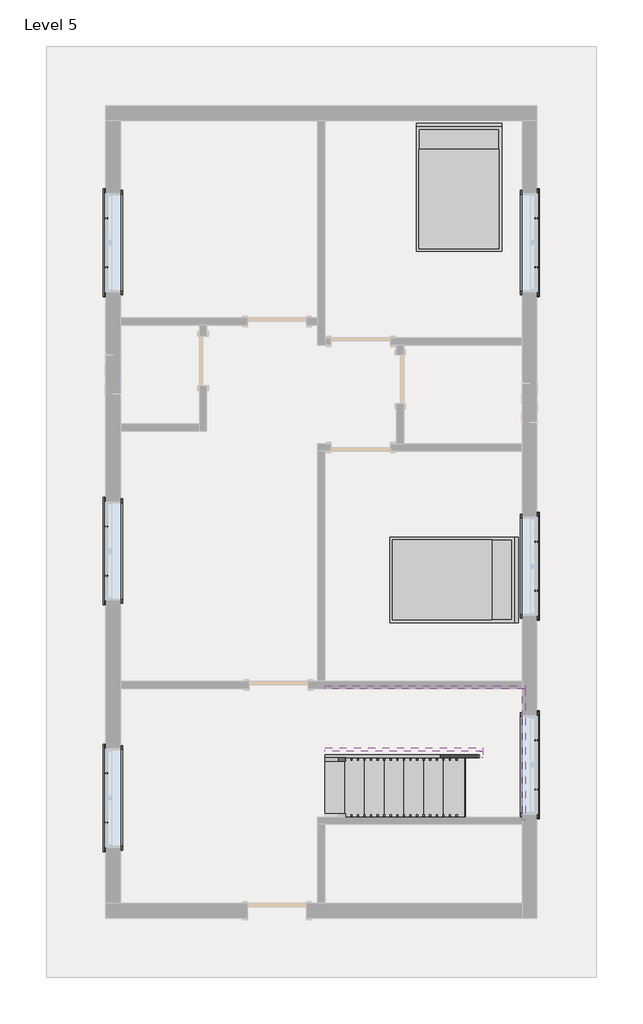
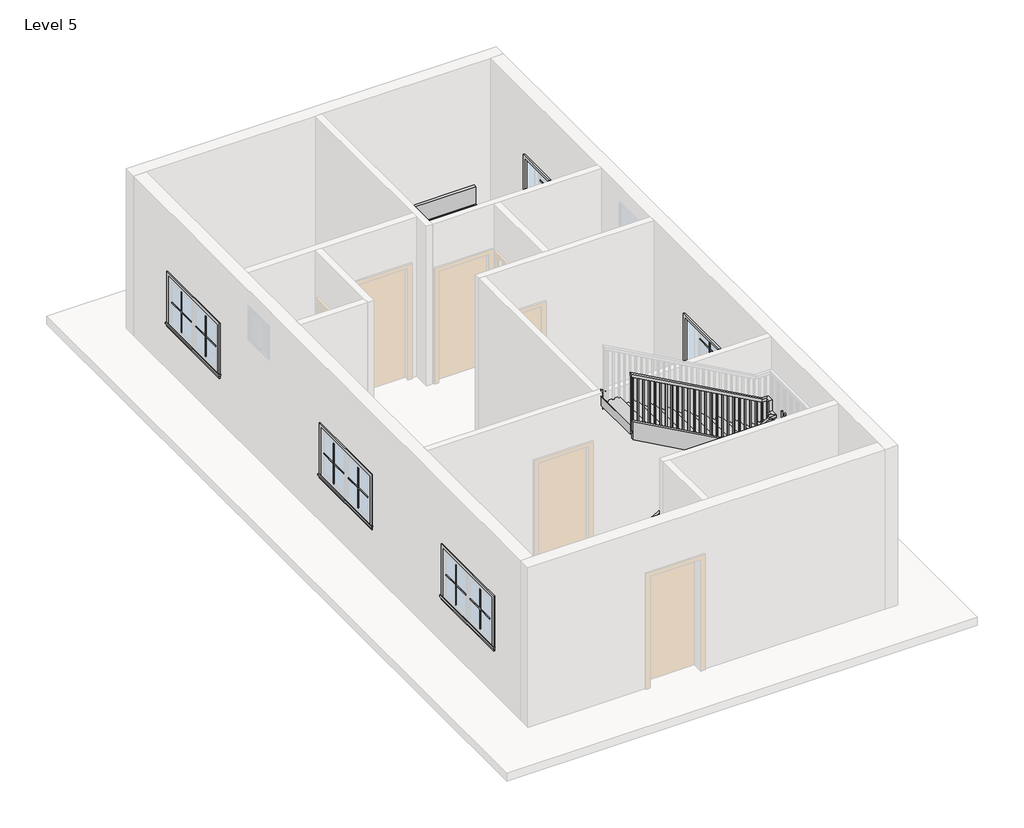
# One storey, part 3 of 3: 24 proxies, 6 members, 2 furniture elements, 1 railing, 1 stair flight.
"""IFC4 building model written with IfcOpenShell, lengths in millimetres."""

from ifc_helpers import new_model, si_unit, frame, origin, place, context, project, spatial, polyline, outline, extrude, faceted_brep, transform, mapped, element, save
from components import muntin_pattern_2x2_muntin_pattern_2x2_9352d081, muntin_pattern_2x2_muntin_pattern_2x2_5c2cbe28, trim_window_exterior_flat_with_sill_979bde60, trim_window_interior_flat_picture_frame_7883d11b, bed_17739_bed_17739_15c61121, stair_flight_c80fa3e3

model = new_model("IFC4")

# Units and contexts
model_context = context("Model", 3, world=origin())
ifc_project = project(units=[si_unit("LENGTHUNIT", "METRE", prefix="MILLI")], contexts=[model_context])

# Site, building, storey
site = spatial("IfcSite", under=ifc_project)
building = spatial("IfcBuilding", under=site)
storey = spatial("IfcBuildingStorey", under=building, Name="Level 5", Elevation=12649.2)

# Proxies
placement = place(None, origin())
muntin_pattern_2x2_muntin_pattern_2x2_shape = muntin_pattern_2x2_muntin_pattern_2x2_9352d081(model_context)
element("IfcBuildingElementProxy", 1, Name="Muntin Pattern_2x2 : Muntin Pattern_2x2", ObjectType="Muntin Pattern_2x2 : Muntin Pattern_2x2", at=placement, inside=storey, context=model_context, shape_type="MappedRepresentation", body=[
    mapped(muntin_pattern_2x2_muntin_pattern_2x2_shape, transform((-4579.34688, 3675.02881, 13633.45), x_axis=(0.0, 1.0, 0.0), y_axis=(-1.0, 0.0, 0.0), z_axis=(0.0, 0.0, 1.0))),
])
element("IfcBuildingElementProxy", 2, Name="Muntin Pattern_2x2 : Muntin Pattern_2x2", ObjectType="Muntin Pattern_2x2 : Muntin Pattern_2x2", at=placement, inside=storey, context=model_context, shape_type="MappedRepresentation", body=[
    mapped(muntin_pattern_2x2_muntin_pattern_2x2_shape, transform((-4579.34688, -1087.47119, 13633.45), x_axis=(0.0, 1.0, 0.0), y_axis=(-1.0, 0.0, 0.0), z_axis=(0.0, 0.0, 1.0))),
])
element("IfcBuildingElementProxy", 3, Name="Muntin Pattern_2x2 : Muntin Pattern_2x2", ObjectType="Muntin Pattern_2x2 : Muntin Pattern_2x2", at=placement, inside=storey, context=model_context, shape_type="MappedRepresentation", body=[
    mapped(muntin_pattern_2x2_muntin_pattern_2x2_shape, transform((-4579.34688, -4900.64619, 13633.45), x_axis=(0.0, 1.0, 0.0), y_axis=(-1.0, 0.0, 0.0), z_axis=(0.0, 0.0, 1.0))),
])
element("IfcBuildingElementProxy", 4, Name="Muntin Pattern_2x2 : Muntin Pattern_2x2", ObjectType="Muntin Pattern_2x2 : Muntin Pattern_2x2", at=placement, inside=storey, context=model_context, shape_type="MappedRepresentation", body=[
    mapped(muntin_pattern_2x2_muntin_pattern_2x2_shape, transform((2069.10312, -3630.64619, 13633.45), x_axis=(0.0, -1.0, 0.0), y_axis=(1.0, 0.0, 0.0), z_axis=(0.0, 0.0, 1.0))),
])
element("IfcBuildingElementProxy", 5, Name="Muntin Pattern_2x2 : Muntin Pattern_2x2", ObjectType="Muntin Pattern_2x2 : Muntin Pattern_2x2", at=placement, inside=storey, context=model_context, shape_type="MappedRepresentation", body=[
    mapped(muntin_pattern_2x2_muntin_pattern_2x2_shape, transform((2069.10312, 4433.85381, 13633.45), x_axis=(0.0, -1.0, 0.0), y_axis=(1.0, 0.0, 0.0), z_axis=(0.0, 0.0, 1.0))),
])
element("IfcBuildingElementProxy", 6, Name="Muntin Pattern_2x2 : Muntin Pattern_2x2", ObjectType="Muntin Pattern_2x2 : Muntin Pattern_2x2", at=placement, inside=storey, context=model_context, shape_type="MappedRepresentation", body=[
    mapped(muntin_pattern_2x2_muntin_pattern_2x2_shape, transform((2069.10312, -563.59619, 13633.45), x_axis=(0.0, -1.0, 0.0), y_axis=(1.0, 0.0, 0.0), z_axis=(0.0, 0.0, 1.0))),
])
muntin_pattern_2x2_muntin_pattern_2x2_2_shape = muntin_pattern_2x2_muntin_pattern_2x2_5c2cbe28(model_context)
element("IfcBuildingElementProxy", 7, Name="Muntin Pattern_2x2 : Muntin Pattern_2x2", ObjectType="Muntin Pattern_2x2 : Muntin Pattern_2x2", at=placement, inside=storey, context=model_context, shape_type="MappedRepresentation", body=[
    mapped(muntin_pattern_2x2_muntin_pattern_2x2_2_shape, transform((-4579.34688, 4433.85381, 13633.45), x_axis=(0.0, -1.0, 0.0), y_axis=(1.0, 0.0, 0.0), z_axis=(0.0, 0.0, 1.0))),
])
element("IfcBuildingElementProxy", 8, Name="Muntin Pattern_2x2 : Muntin Pattern_2x2", ObjectType="Muntin Pattern_2x2 : Muntin Pattern_2x2", at=placement, inside=storey, context=model_context, shape_type="MappedRepresentation", body=[
    mapped(muntin_pattern_2x2_muntin_pattern_2x2_2_shape, transform((-4579.34688, -328.64619, 13633.45), x_axis=(0.0, -1.0, 0.0), y_axis=(1.0, 0.0, 0.0), z_axis=(0.0, 0.0, 1.0))),
])
element("IfcBuildingElementProxy", 9, Name="Muntin Pattern_2x2 : Muntin Pattern_2x2", ObjectType="Muntin Pattern_2x2 : Muntin Pattern_2x2", at=placement, inside=storey, context=model_context, shape_type="MappedRepresentation", body=[
    mapped(muntin_pattern_2x2_muntin_pattern_2x2_2_shape, transform((-4579.34688, -4141.82119, 13633.45), x_axis=(0.0, -1.0, 0.0), y_axis=(1.0, 0.0, 0.0), z_axis=(0.0, 0.0, 1.0))),
])
element("IfcBuildingElementProxy", 10, Name="Muntin Pattern_2x2 : Muntin Pattern_2x2", ObjectType="Muntin Pattern_2x2 : Muntin Pattern_2x2", at=placement, inside=storey, context=model_context, shape_type="MappedRepresentation", body=[
    mapped(muntin_pattern_2x2_muntin_pattern_2x2_2_shape, transform((2069.10312, -4389.47119, 13633.45), x_axis=(0.0, 1.0, 0.0), y_axis=(-1.0, 0.0, 0.0), z_axis=(0.0, 0.0, 1.0))),
])
element("IfcBuildingElementProxy", 11, Name="Muntin Pattern_2x2 : Muntin Pattern_2x2", ObjectType="Muntin Pattern_2x2 : Muntin Pattern_2x2", at=placement, inside=storey, context=model_context, shape_type="MappedRepresentation", body=[
    mapped(muntin_pattern_2x2_muntin_pattern_2x2_2_shape, transform((2069.10312, 3675.02881, 13633.45), x_axis=(0.0, 1.0, 0.0), y_axis=(-1.0, 0.0, 0.0), z_axis=(0.0, 0.0, 1.0))),
])
element("IfcBuildingElementProxy", 12, Name="Muntin Pattern_2x2 : Muntin Pattern_2x2", ObjectType="Muntin Pattern_2x2 : Muntin Pattern_2x2", at=placement, inside=storey, context=model_context, shape_type="MappedRepresentation", body=[
    mapped(muntin_pattern_2x2_muntin_pattern_2x2_2_shape, transform((2069.10312, -1322.42119, 13633.45), x_axis=(0.0, 1.0, 0.0), y_axis=(-1.0, 0.0, 0.0), z_axis=(0.0, 0.0, 1.0))),
])
trim_window_exterior_flat_with_sill_shape = trim_window_exterior_flat_with_sill_979bde60(model_context)
element("IfcBuildingElementProxy", 13, Name="Trim-Window-Exterior-Flat : with Sill", ObjectType="Trim-Window-Exterior-Flat : with Sill", at=placement, inside=storey, context=model_context, shape_type="MappedRepresentation", body=[
    mapped(trim_window_exterior_flat_with_sill_shape, transform((-4588.87188, 4054.44131, 14478.0), x_axis=(0.0, -1.0, 0.0), y_axis=(0.0, 0.0, 1.0), z_axis=(-1.0, 0.0, 0.0))),
])
element("IfcBuildingElementProxy", 14, Name="Trim-Window-Exterior-Flat : with Sill", ObjectType="Trim-Window-Exterior-Flat : with Sill", at=placement, inside=storey, context=model_context, shape_type="MappedRepresentation", body=[
    mapped(trim_window_exterior_flat_with_sill_shape, transform((-4588.87188, -708.05869, 14478.0), x_axis=(0.0, -1.0, 0.0), y_axis=(0.0, 0.0, 1.0), z_axis=(-1.0, 0.0, 0.0))),
])
element("IfcBuildingElementProxy", 15, Name="Trim-Window-Exterior-Flat : with Sill", ObjectType="Trim-Window-Exterior-Flat : with Sill", at=placement, inside=storey, context=model_context, shape_type="MappedRepresentation", body=[
    mapped(trim_window_exterior_flat_with_sill_shape, transform((-4588.87188, -4521.23369, 14478.0), x_axis=(0.0, -1.0, 0.0), y_axis=(0.0, 0.0, 1.0), z_axis=(-1.0, 0.0, 0.0))),
])
element("IfcBuildingElementProxy", 16, Name="Trim-Window-Exterior-Flat : with Sill", ObjectType="Trim-Window-Exterior-Flat : with Sill", at=placement, inside=storey, context=model_context, shape_type="MappedRepresentation", body=[
    mapped(trim_window_exterior_flat_with_sill_shape, transform((2078.62812, -4010.05869, 14478.0), x_axis=(0.0, 1.0, 0.0), y_axis=(0.0, 0.0, 1.0), z_axis=(1.0, 0.0, 0.0))),
])
element("IfcBuildingElementProxy", 17, Name="Trim-Window-Exterior-Flat : with Sill", ObjectType="Trim-Window-Exterior-Flat : with Sill", at=placement, inside=storey, context=model_context, shape_type="MappedRepresentation", body=[
    mapped(trim_window_exterior_flat_with_sill_shape, transform((2078.62812, 4054.44131, 14478.0), x_axis=(0.0, 1.0, 0.0), y_axis=(0.0, 0.0, 1.0), z_axis=(1.0, 0.0, 0.0))),
])
element("IfcBuildingElementProxy", 18, Name="Trim-Window-Exterior-Flat : with Sill", ObjectType="Trim-Window-Exterior-Flat : with Sill", at=placement, inside=storey, context=model_context, shape_type="MappedRepresentation", body=[
    mapped(trim_window_exterior_flat_with_sill_shape, transform((2078.62812, -943.00869, 14478.0), x_axis=(0.0, 1.0, 0.0), y_axis=(0.0, 0.0, 1.0), z_axis=(1.0, 0.0, 0.0))),
])
trim_window_interior_flat_picture_frame_shape = trim_window_interior_flat_picture_frame_7883d11b(model_context)
element("IfcBuildingElementProxy", 19, Name="Trim-Window-Interior-Flat : Picture Frame", ObjectType="Trim-Window-Interior-Flat : Picture Frame", at=placement, inside=storey, context=model_context, shape_type="MappedRepresentation", body=[
    mapped(trim_window_interior_flat_picture_frame_shape, transform((-4360.27188, 4054.44131, 14478.0), x_axis=(0.0, 1.0, 0.0), y_axis=(0.0, 0.0, 1.0), z_axis=(1.0, 0.0, 0.0))),
])
element("IfcBuildingElementProxy", 20, Name="Trim-Window-Interior-Flat : Picture Frame", ObjectType="Trim-Window-Interior-Flat : Picture Frame", at=placement, inside=storey, context=model_context, shape_type="MappedRepresentation", body=[
    mapped(trim_window_interior_flat_picture_frame_shape, transform((-4360.27188, -708.05869, 14478.0), x_axis=(0.0, 1.0, 0.0), y_axis=(0.0, 0.0, 1.0), z_axis=(1.0, 0.0, 0.0))),
])
element("IfcBuildingElementProxy", 21, Name="Trim-Window-Interior-Flat : Picture Frame", ObjectType="Trim-Window-Interior-Flat : Picture Frame", at=placement, inside=storey, context=model_context, shape_type="MappedRepresentation", body=[
    mapped(trim_window_interior_flat_picture_frame_shape, transform((-4360.27188, -4521.23369, 14478.0), x_axis=(0.0, 1.0, 0.0), y_axis=(0.0, 0.0, 1.0), z_axis=(1.0, 0.0, 0.0))),
])
element("IfcBuildingElementProxy", 22, Name="Trim-Window-Interior-Flat : Picture Frame", ObjectType="Trim-Window-Interior-Flat : Picture Frame", at=placement, inside=storey, context=model_context, shape_type="MappedRepresentation", body=[
    mapped(trim_window_interior_flat_picture_frame_shape, transform((1850.02812, -4010.05869, 14478.0), x_axis=(0.0, -1.0, 0.0), y_axis=(0.0, 0.0, 1.0), z_axis=(-1.0, 0.0, 0.0))),
])
element("IfcBuildingElementProxy", 23, Name="Trim-Window-Interior-Flat : Picture Frame", ObjectType="Trim-Window-Interior-Flat : Picture Frame", at=placement, inside=storey, context=model_context, shape_type="MappedRepresentation", body=[
    mapped(trim_window_interior_flat_picture_frame_shape, transform((1850.02812, 4054.44131, 14478.0), x_axis=(0.0, -1.0, 0.0), y_axis=(0.0, 0.0, 1.0), z_axis=(-1.0, 0.0, 0.0))),
])
element("IfcBuildingElementProxy", 24, Name="Trim-Window-Interior-Flat : Picture Frame", ObjectType="Trim-Window-Interior-Flat : Picture Frame", at=placement, inside=storey, context=model_context, shape_type="MappedRepresentation", body=[
    mapped(trim_window_interior_flat_picture_frame_shape, transform((1850.02812, -943.00869, 14478.0), x_axis=(0.0, -1.0, 0.0), y_axis=(0.0, 0.0, 1.0), z_axis=(-1.0, 0.0, 0.0))),
])

# Furniture
bed_17739_bed_17739_shape = bed_17739_bed_17739_15c61121(model_context)
element("IfcFurniture", 25, ObjectType="Bed_17739 : Bed_17739", at=placement, inside=storey, context=model_context, shape_type="MappedRepresentation", body=[
    mapped(bed_17739_bed_17739_shape, transform((872.12812, 4886.29131, 12649.2), x_axis=(1.0, 0.0, 0.0), y_axis=(0.0, 1.0, 0.0), z_axis=(0.0, 0.0, 1.0))),
])
element("IfcFurniture", 26, ObjectType="Bed_17739 : Bed_17739", at=placement, inside=storey, context=model_context, shape_type="MappedRepresentation", body=[
    mapped(bed_17739_bed_17739_shape, transform((770.52812, -1152.55869, 12649.2), x_axis=(0.0, -1.0, 0.0), y_axis=(1.0, 0.0, 0.0), z_axis=(0.0, 0.0, 1.0))),
])

# Members
element("IfcMember", 27, ObjectType="Stringer - 2\" Width", at=placement, inside=storey, context=model_context, shape_type="SweptSolid", body=[
    extrude(outline(polyline([(12856.7983948, -1197.97188), (12649.2, -1197.97188), (12649.2, -944.0273772), (13834.5641651, 1189.62812), (14183.2428392, 1189.62812), (12856.7983948, -1197.97188)])), frame((0.0, -3902.10869, 0.0), z_axis=(0.0, 1.0, 0.0), x_axis=(0.0, 0.0, 1.0)), (0.0, 0.0, 1.0), 50.8),
])
element("IfcMember", 28, ObjectType="Stringer - 2\" Width", at=placement, inside=storey, context=model_context, shape_type="SweptSolid", body=[
    extrude(outline(polyline([(1240.42812, -3902.10869), (1189.62812, -3902.10869), (1189.62812, -3800.50869), (1240.42812, -3800.50869), (1240.42812, -3902.10869)])), frame((0.0, 0.0, 13944.6), z_axis=(0.0, 0.0, 1.0), x_axis=(1.0, 0.0, 0.0)), (0.0, 0.0, 1.0), 304.8),
])
element("IfcMember", 29, ObjectType="Stringer - 2\" Width", at=placement, inside=storey, context=model_context, shape_type="SweptSolid", body=[
    extrude(outline(polyline([(14032.1197207, 1240.42812), (14380.7983948, 1240.42812), (15735.4650614, -1197.97188), (15386.7863873, -1197.97188), (14032.1197207, 1240.42812)])), frame((0.0, -3800.50869, 0.0), z_axis=(0.0, 1.0, 0.0), x_axis=(0.0, 0.0, 1.0)), (0.0, 0.0, 1.0), 50.8),
])
element("IfcMember", 30, ObjectType="Stringer - 2\" Width", at=placement, inside=storey, context=model_context, shape_type="SweptSolid", body=[
    extrude(outline(polyline([(12856.7983948, -1197.97188), (12649.2, -1197.97188), (12649.2, -944.0273772), (14201.453054, 1850.02812), (14249.4, 1850.02812), (14249.4, 1308.7110094), (12856.7983948, -1197.97188)])), frame((0.0, -4867.30869, 0.0), z_axis=(0.0, 1.0, 0.0), x_axis=(0.0, 0.0, 1.0)), (0.0, 0.0, 1.0), 50.8),
])
element("IfcMember", 31, ObjectType="Stringer - 2\" Width", at=placement, inside=storey, context=model_context, shape_type="SweptSolid", body=[
    extrude(outline(polyline([(1900.82812, -4867.30869), (1850.02812, -4867.30869), (1850.02812, -2835.30869), (1900.82812, -2835.30869), (1900.82812, -4867.30869)])), frame((0.0, 0.0, 13944.6), z_axis=(0.0, 0.0, 1.0), x_axis=(1.0, 0.0, 0.0)), (0.0, 0.0, 1.0), 304.8),
])
element("IfcMember", 32, ObjectType="Stringer - 2\" Width", at=placement, inside=storey, context=model_context, shape_type="SweptSolid", body=[
    extrude(outline(polyline([(13944.6, 1900.82812), (14013.9095059, 1900.82812), (15735.4650614, -1197.97188), (15386.7863873, -1197.97188), (13944.6, 1397.9636172), (13944.6, 1900.82812)])), frame((0.0, -2835.30869, 0.0), z_axis=(0.0, 1.0, 0.0), x_axis=(0.0, 0.0, 1.0)), (0.0, 0.0, 1.0), 50.8),
])

# Railing
element("IfcRailing", 33, ObjectType="Handrail - Rectangular", at=placement, inside=storey, context=model_context, shape_type="SolidModel", body=[
    faceted_brep([(-1197.97188, -3902.10869, 13732.9333333), (-1197.97188, -3902.10869, 13674.820221), (-1197.97188, -3952.90869, 13674.820221), (-1197.97188, -3952.90869, 13732.9333333), (1164.22812, -3902.10869, 15045.2666667), (1215.02812, -3902.10869, 15015.3757765), (1215.02812, -3952.90869, 15015.3757765), (1164.22812, -3952.90869, 15045.2666667), (1164.22812, -3902.10869, 15087.6), (1215.02812, -3902.10869, 15036.8), (1215.02812, -3952.90869, 15036.8), (1164.22812, -3952.90869, 15087.6), (1240.42812, -3902.10869, 15087.6), (1240.42812, -3902.10869, 15036.8), (1291.22812, -3952.90869, 15036.8), (1291.22812, -3952.90869, 15087.6), (1240.42812, -3825.90869, 15087.6), (1240.42812, -3775.10869, 15036.8), (1291.22812, -3775.10869, 15036.8), (1291.22812, -3825.90869, 15087.6), (1240.42812, -3825.90869, 15299.2666667), (1240.42812, -3775.10869, 15248.4666667), (1291.22812, -3775.10869, 15248.4666667), (1291.22812, -3825.90869, 15299.2666667), (1240.42812, -3749.70869, 15299.2666667), (1240.42812, -3749.70869, 15248.4666667), (1291.22812, -3698.90869, 15248.4666667), (1291.22812, -3698.90869, 15299.2666667), (1164.22812, -3749.70869, 15299.2666667), (1151.0645177, -3749.70869, 15248.4666667), (1151.0645177, -3698.90869, 15248.4666667), (1164.22812, -3698.90869, 15299.2666667), (-1197.97188, -3749.70869, 16611.6), (-1197.97188, -3698.90869, 16611.6), (-1197.97188, -3698.90869, 16553.4868876), (-1197.97188, -3749.70869, 16553.4868876)], [[[0, 1, 2, 3]], [[1, 0, 4, 5]], [[2, 1, 5, 6]], [[3, 2, 6, 7]], [[0, 3, 7, 4]], [[5, 4, 8, 9]], [[6, 5, 9, 10]], [[7, 6, 10, 11]], [[4, 7, 11, 8]], [[9, 8, 12, 13]], [[10, 9, 13, 14]], [[11, 10, 14, 15]], [[8, 11, 15, 12]], [[13, 12, 16, 17]], [[14, 13, 17, 18]], [[15, 14, 18, 19]], [[12, 15, 19, 16]], [[17, 16, 20, 21]], [[18, 17, 21, 22]], [[19, 18, 22, 23]], [[16, 19, 23, 20]], [[21, 20, 24, 25]], [[22, 21, 25, 26]], [[23, 22, 26, 27]], [[20, 23, 27, 24]], [[25, 24, 28, 29]], [[26, 25, 29, 30]], [[27, 26, 30, 31]], [[24, 27, 31, 28]], [[32, 33, 34, 35]], [[29, 28, 32, 35]], [[30, 29, 35, 34]], [[31, 30, 34, 33]], [[28, 31, 33, 32]]]),
    extrude(outline(polyline([(16544.6674432, -1182.09688), (15527.8666667, -1182.09688), (15527.8666667, -1163.04688), (16534.0841099, -1163.04688), (16544.6674432, -1182.09688)])), frame((0.0, -3733.83369, 0.0), z_axis=(0.0, 1.0, 0.0), x_axis=(0.0, 0.0, 1.0)), (0.0, 0.0, 1.0), 19.05),
    extrude(outline(polyline([(16488.2229988, -1080.49688), (15527.8666667, -1080.49688), (15527.8666667, -1061.44688), (16477.6396654, -1061.44688), (16488.2229988, -1080.49688)])), frame((0.0, -3733.83369, 0.0), z_axis=(0.0, 1.0, 0.0), x_axis=(0.0, 0.0, 1.0)), (0.0, 0.0, 1.0), 19.05),
    extrude(outline(polyline([(16431.7785543, -978.89688), (15527.8666667, -978.89688), (15527.8666667, -959.84688), (16421.195221, -959.84688), (16431.7785543, -978.89688)])), frame((0.0, -3733.83369, 0.0), z_axis=(0.0, 1.0, 0.0), x_axis=(0.0, 0.0, 1.0)), (0.0, 0.0, 1.0), 19.05),
    extrude(outline(polyline([(16375.3341099, -877.29688), (15358.5333333, -877.29688), (15358.5333333, -858.24688), (16364.7507765, -858.24688), (16375.3341099, -877.29688)])), frame((0.0, -3733.83369, 0.0), z_axis=(0.0, 1.0, 0.0), x_axis=(0.0, 0.0, 1.0)), (0.0, 0.0, 1.0), 19.05),
    extrude(outline(polyline([(16318.8896654, -775.69688), (15358.5333333, -775.69688), (15358.5333333, -756.64688), (16308.3063321, -756.64688), (16318.8896654, -775.69688)])), frame((0.0, -3733.83369, 0.0), z_axis=(0.0, 1.0, 0.0), x_axis=(0.0, 0.0, 1.0)), (0.0, 0.0, 1.0), 19.05),
    extrude(outline(polyline([(16262.445221, -674.09688), (15358.5333333, -674.09688), (15358.5333333, -655.04688), (16251.8618876, -655.04688), (16262.445221, -674.09688)])), frame((0.0, -3733.83369, 0.0), z_axis=(0.0, 1.0, 0.0), x_axis=(0.0, 0.0, 1.0)), (0.0, 0.0, 1.0), 19.05),
    extrude(outline(polyline([(16206.0007765, -572.49688), (15189.2, -572.49688), (15189.2, -553.44688), (16195.4174432, -553.44688), (16206.0007765, -572.49688)])), frame((0.0, -3733.83369, 0.0), z_axis=(0.0, 1.0, 0.0), x_axis=(0.0, 0.0, 1.0)), (0.0, 0.0, 1.0), 19.05),
    extrude(outline(polyline([(16149.5563321, -470.89688), (15189.2, -470.89688), (15189.2, -451.84688), (16138.9729988, -451.84688), (16149.5563321, -470.89688)])), frame((0.0, -3733.83369, 0.0), z_axis=(0.0, 1.0, 0.0), x_axis=(0.0, 0.0, 1.0)), (0.0, 0.0, 1.0), 19.05),
    extrude(outline(polyline([(16093.1118876, -369.29688), (15189.2, -369.29688), (15189.2, -350.24688), (16082.5285543, -350.24688), (16093.1118876, -369.29688)])), frame((0.0, -3733.83369, 0.0), z_axis=(0.0, 1.0, 0.0), x_axis=(0.0, 0.0, 1.0)), (0.0, 0.0, 1.0), 19.05),
    extrude(outline(polyline([(16036.6674432, -267.69688), (15019.8666667, -267.69688), (15019.8666667, -248.64688), (16026.0841099, -248.64688), (16036.6674432, -267.69688)])), frame((0.0, -3733.83369, 0.0), z_axis=(0.0, 1.0, 0.0), x_axis=(0.0, 0.0, 1.0)), (0.0, 0.0, 1.0), 19.05),
    extrude(outline(polyline([(15980.2229988, -166.09688), (15019.8666667, -166.09688), (15019.8666667, -147.04688), (15969.6396654, -147.04688), (15980.2229988, -166.09688)])), frame((0.0, -3733.83369, 0.0), z_axis=(0.0, 1.0, 0.0), x_axis=(0.0, 0.0, 1.0)), (0.0, 0.0, 1.0), 19.05),
    extrude(outline(polyline([(15923.7785543, -64.49688), (15019.8666667, -64.49688), (15019.8666667, -45.44688), (15913.195221, -45.44688), (15923.7785543, -64.49688)])), frame((0.0, -3733.83369, 0.0), z_axis=(0.0, 1.0, 0.0), x_axis=(0.0, 0.0, 1.0)), (0.0, 0.0, 1.0), 19.05),
    extrude(outline(polyline([(15867.3341099, 37.10312), (14850.5333333, 37.10312), (14850.5333333, 56.15312), (15856.7507765, 56.15312), (15867.3341099, 37.10312)])), frame((0.0, -3733.83369, 0.0), z_axis=(0.0, 1.0, 0.0), x_axis=(0.0, 0.0, 1.0)), (0.0, 0.0, 1.0), 19.05),
    extrude(outline(polyline([(15810.8896654, 138.70312), (14850.5333333, 138.70312), (14850.5333333, 157.75312), (15800.3063321, 157.75312), (15810.8896654, 138.70312)])), frame((0.0, -3733.83369, 0.0), z_axis=(0.0, 1.0, 0.0), x_axis=(0.0, 0.0, 1.0)), (0.0, 0.0, 1.0), 19.05),
    extrude(outline(polyline([(15754.445221, 240.30312), (14850.5333333, 240.30312), (14850.5333333, 259.35312), (15743.8618876, 259.35312), (15754.445221, 240.30312)])), frame((0.0, -3733.83369, 0.0), z_axis=(0.0, 1.0, 0.0), x_axis=(0.0, 0.0, 1.0)), (0.0, 0.0, 1.0), 19.05),
    extrude(outline(polyline([(15698.0007765, 341.90312), (14681.2, 341.90312), (14681.2, 360.95312), (15687.4174432, 360.95312), (15698.0007765, 341.90312)])), frame((0.0, -3733.83369, 0.0), z_axis=(0.0, 1.0, 0.0), x_axis=(0.0, 0.0, 1.0)), (0.0, 0.0, 1.0), 19.05),
    extrude(outline(polyline([(15641.5563321, 443.50312), (14681.2, 443.50312), (14681.2, 462.55312), (15630.9729988, 462.55312), (15641.5563321, 443.50312)])), frame((0.0, -3733.83369, 0.0), z_axis=(0.0, 1.0, 0.0), x_axis=(0.0, 0.0, 1.0)), (0.0, 0.0, 1.0), 19.05),
    extrude(outline(polyline([(15585.1118876, 545.10312), (14681.2, 545.10312), (14681.2, 564.15312), (15574.5285543, 564.15312), (15585.1118876, 545.10312)])), frame((0.0, -3733.83369, 0.0), z_axis=(0.0, 1.0, 0.0), x_axis=(0.0, 0.0, 1.0)), (0.0, 0.0, 1.0), 19.05),
    extrude(outline(polyline([(15528.6674432, 646.70312), (14511.8666667, 646.70312), (14511.8666667, 665.75312), (15518.0841099, 665.75312), (15528.6674432, 646.70312)])), frame((0.0, -3733.83369, 0.0), z_axis=(0.0, 1.0, 0.0), x_axis=(0.0, 0.0, 1.0)), (0.0, 0.0, 1.0), 19.05),
    extrude(outline(polyline([(15472.2229988, 748.30312), (14511.8666667, 748.30312), (14511.8666667, 767.35312), (15461.6396654, 767.35312), (15472.2229988, 748.30312)])), frame((0.0, -3733.83369, 0.0), z_axis=(0.0, 1.0, 0.0), x_axis=(0.0, 0.0, 1.0)), (0.0, 0.0, 1.0), 19.05),
    extrude(outline(polyline([(15415.7785543, 849.90312), (14511.8666667, 849.90312), (14511.8666667, 868.95312), (15405.195221, 868.95312), (15415.7785543, 849.90312)])), frame((0.0, -3733.83369, 0.0), z_axis=(0.0, 1.0, 0.0), x_axis=(0.0, 0.0, 1.0)), (0.0, 0.0, 1.0), 19.05),
    extrude(outline(polyline([(15359.3341099, 951.50312), (14342.5333333, 951.50312), (14342.5333333, 970.55312), (15348.7507765, 970.55312), (15359.3341099, 951.50312)])), frame((0.0, -3733.83369, 0.0), z_axis=(0.0, 1.0, 0.0), x_axis=(0.0, 0.0, 1.0)), (0.0, 0.0, 1.0), 19.05),
    extrude(outline(polyline([(15302.8896654, 1053.10312), (14342.5333333, 1053.10312), (14342.5333333, 1072.15312), (15292.3063321, 1072.15312), (15302.8896654, 1053.10312)])), frame((0.0, -3733.83369, 0.0), z_axis=(0.0, 1.0, 0.0), x_axis=(0.0, 0.0, 1.0)), (0.0, 0.0, 1.0), 19.05),
    extrude(outline(polyline([(15246.445221, 1154.70312), (14342.5333333, 1154.70312), (14342.5333333, 1173.75312), (15235.8618876, 1173.75312), (15246.445221, 1154.70312)])), frame((0.0, -3733.83369, 0.0), z_axis=(0.0, 1.0, 0.0), x_axis=(0.0, 0.0, 1.0)), (0.0, 0.0, 1.0), 19.05),
    extrude(outline(polyline([(1256.30312, -3835.43369), (1256.30312, -3816.38369), (1275.35312, -3816.38369), (1275.35312, -3835.43369), (1256.30312, -3835.43369)])), frame((0.0, 0.0, 14173.2), z_axis=(0.0, 0.0, 1.0), x_axis=(1.0, 0.0, 0.0)), (0.0, 0.0, 1.0), 863.6),
    extrude(outline(polyline([(1230.90312, -3917.98369), (1249.95312, -3917.98369), (1249.95312, -3937.03369), (1230.90312, -3937.03369), (1230.90312, -3917.98369)])), frame((0.0, 0.0, 14173.2), z_axis=(0.0, 0.0, 1.0), x_axis=(1.0, 0.0, 0.0)), (0.0, 0.0, 1.0), 863.6),
    extrude(outline(polyline([(14967.7507765, 1129.30312), (14003.8666667, 1129.30312), (14003.8666667, 1148.35312), (14978.3341099, 1148.35312), (14967.7507765, 1129.30312)])), frame((0.0, -3937.03369, 0.0), z_axis=(0.0, 1.0, 0.0), x_axis=(0.0, 0.0, 1.0)), (0.0, 0.0, 1.0), 19.05),
    extrude(outline(polyline([(14911.3063321, 1027.70312), (14003.8666667, 1027.70312), (14003.8666667, 1046.75312), (14921.8896654, 1046.75312), (14911.3063321, 1027.70312)])), frame((0.0, -3937.03369, 0.0), z_axis=(0.0, 1.0, 0.0), x_axis=(0.0, 0.0, 1.0)), (0.0, 0.0, 1.0), 19.05),
    extrude(outline(polyline([(14854.8618876, 926.10312), (14003.8666667, 926.10312), (14003.8666667, 945.15312), (14865.445221, 945.15312), (14854.8618876, 926.10312)])), frame((0.0, -3937.03369, 0.0), z_axis=(0.0, 1.0, 0.0), x_axis=(0.0, 0.0, 1.0)), (0.0, 0.0, 1.0), 19.05),
    extrude(outline(polyline([(14798.4174432, 824.50312), (13834.5333333, 824.50312), (13834.5333333, 843.55312), (14809.0007765, 843.55312), (14798.4174432, 824.50312)])), frame((0.0, -3937.03369, 0.0), z_axis=(0.0, 1.0, 0.0), x_axis=(0.0, 0.0, 1.0)), (0.0, 0.0, 1.0), 19.05),
    extrude(outline(polyline([(14741.9729988, 722.90312), (13834.5333333, 722.90312), (13834.5333333, 741.95312), (14752.5563321, 741.95312), (14741.9729988, 722.90312)])), frame((0.0, -3937.03369, 0.0), z_axis=(0.0, 1.0, 0.0), x_axis=(0.0, 0.0, 1.0)), (0.0, 0.0, 1.0), 19.05),
    extrude(outline(polyline([(14685.5285543, 621.30312), (13834.5333333, 621.30312), (13834.5333333, 640.35312), (14696.1118876, 640.35312), (14685.5285543, 621.30312)])), frame((0.0, -3937.03369, 0.0), z_axis=(0.0, 1.0, 0.0), x_axis=(0.0, 0.0, 1.0)), (0.0, 0.0, 1.0), 19.05),
    extrude(outline(polyline([(14629.0841099, 519.70312), (13665.2, 519.70312), (13665.2, 538.75312), (14639.6674432, 538.75312), (14629.0841099, 519.70312)])), frame((0.0, -3937.03369, 0.0), z_axis=(0.0, 1.0, 0.0), x_axis=(0.0, 0.0, 1.0)), (0.0, 0.0, 1.0), 19.05),
    extrude(outline(polyline([(14572.6396654, 418.10312), (13665.2, 418.10312), (13665.2, 437.15312), (14583.2229988, 437.15312), (14572.6396654, 418.10312)])), frame((0.0, -3937.03369, 0.0), z_axis=(0.0, 1.0, 0.0), x_axis=(0.0, 0.0, 1.0)), (0.0, 0.0, 1.0), 19.05),
    extrude(outline(polyline([(14516.195221, 316.50312), (13665.2, 316.50312), (13665.2, 335.55312), (14526.7785543, 335.55312), (14516.195221, 316.50312)])), frame((0.0, -3937.03369, 0.0), z_axis=(0.0, 1.0, 0.0), x_axis=(0.0, 0.0, 1.0)), (0.0, 0.0, 1.0), 19.05),
    extrude(outline(polyline([(14459.7507765, 214.90312), (13495.8666667, 214.90312), (13495.8666667, 233.95312), (14470.3341099, 233.95312), (14459.7507765, 214.90312)])), frame((0.0, -3937.03369, 0.0), z_axis=(0.0, 1.0, 0.0), x_axis=(0.0, 0.0, 1.0)), (0.0, 0.0, 1.0), 19.05),
    extrude(outline(polyline([(14403.3063321, 113.30312), (13495.8666667, 113.30312), (13495.8666667, 132.35312), (14413.8896654, 132.35312), (14403.3063321, 113.30312)])), frame((0.0, -3937.03369, 0.0), z_axis=(0.0, 1.0, 0.0), x_axis=(0.0, 0.0, 1.0)), (0.0, 0.0, 1.0), 19.05),
    extrude(outline(polyline([(14346.8618876, 11.70312), (13495.8666667, 11.70312), (13495.8666667, 30.75312), (14357.445221, 30.75312), (14346.8618876, 11.70312)])), frame((0.0, -3937.03369, 0.0), z_axis=(0.0, 1.0, 0.0), x_axis=(0.0, 0.0, 1.0)), (0.0, 0.0, 1.0), 19.05),
    extrude(outline(polyline([(14290.4174432, -89.89688), (13326.5333333, -89.89688), (13326.5333333, -70.84688), (14301.0007765, -70.84688), (14290.4174432, -89.89688)])), frame((0.0, -3937.03369, 0.0), z_axis=(0.0, 1.0, 0.0), x_axis=(0.0, 0.0, 1.0)), (0.0, 0.0, 1.0), 19.05),
    extrude(outline(polyline([(14233.9729988, -191.49688), (13326.5333333, -191.49688), (13326.5333333, -172.44688), (14244.5563321, -172.44688), (14233.9729988, -191.49688)])), frame((0.0, -3937.03369, 0.0), z_axis=(0.0, 1.0, 0.0), x_axis=(0.0, 0.0, 1.0)), (0.0, 0.0, 1.0), 19.05),
    extrude(outline(polyline([(14177.5285543, -293.09688), (13326.5333333, -293.09688), (13326.5333333, -274.04688), (14188.1118876, -274.04688), (14177.5285543, -293.09688)])), frame((0.0, -3937.03369, 0.0), z_axis=(0.0, 1.0, 0.0), x_axis=(0.0, 0.0, 1.0)), (0.0, 0.0, 1.0), 19.05),
    extrude(outline(polyline([(14121.0841099, -394.69688), (13157.2, -394.69688), (13157.2, -375.64688), (14131.6674432, -375.64688), (14121.0841099, -394.69688)])), frame((0.0, -3937.03369, 0.0), z_axis=(0.0, 1.0, 0.0), x_axis=(0.0, 0.0, 1.0)), (0.0, 0.0, 1.0), 19.05),
    extrude(outline(polyline([(14064.6396654, -496.29688), (13157.2, -496.29688), (13157.2, -477.24688), (14075.2229988, -477.24688), (14064.6396654, -496.29688)])), frame((0.0, -3937.03369, 0.0), z_axis=(0.0, 1.0, 0.0), x_axis=(0.0, 0.0, 1.0)), (0.0, 0.0, 1.0), 19.05),
    extrude(outline(polyline([(14008.195221, -597.89688), (13157.2, -597.89688), (13157.2, -578.84688), (14018.7785543, -578.84688), (14008.195221, -597.89688)])), frame((0.0, -3937.03369, 0.0), z_axis=(0.0, 1.0, 0.0), x_axis=(0.0, 0.0, 1.0)), (0.0, 0.0, 1.0), 19.05),
    extrude(outline(polyline([(13951.7507765, -699.49688), (12987.8666667, -699.49688), (12987.8666667, -680.44688), (13962.3341099, -680.44688), (13951.7507765, -699.49688)])), frame((0.0, -3937.03369, 0.0), z_axis=(0.0, 1.0, 0.0), x_axis=(0.0, 0.0, 1.0)), (0.0, 0.0, 1.0), 19.05),
    extrude(outline(polyline([(13895.3063321, -801.09688), (12987.8666667, -801.09688), (12987.8666667, -782.04688), (13905.8896654, -782.04688), (13895.3063321, -801.09688)])), frame((0.0, -3937.03369, 0.0), z_axis=(0.0, 1.0, 0.0), x_axis=(0.0, 0.0, 1.0)), (0.0, 0.0, 1.0), 19.05),
    extrude(outline(polyline([(13838.8618876, -902.69688), (12987.8666667, -902.69688), (12987.8666667, -883.64688), (13849.445221, -883.64688), (13838.8618876, -902.69688)])), frame((0.0, -3937.03369, 0.0), z_axis=(0.0, 1.0, 0.0), x_axis=(0.0, 0.0, 1.0)), (0.0, 0.0, 1.0), 19.05),
    extrude(outline(polyline([(13782.4174432, -1004.29688), (12818.5333333, -1004.29688), (12818.5333333, -985.24688), (13793.0007765, -985.24688), (13782.4174432, -1004.29688)])), frame((0.0, -3937.03369, 0.0), z_axis=(0.0, 1.0, 0.0), x_axis=(0.0, 0.0, 1.0)), (0.0, 0.0, 1.0), 19.05),
    extrude(outline(polyline([(13725.9729988, -1105.89688), (12818.5333333, -1105.89688), (12818.5333333, -1086.84688), (13736.5563321, -1086.84688), (13725.9729988, -1105.89688)])), frame((0.0, -3937.03369, 0.0), z_axis=(0.0, 1.0, 0.0), x_axis=(0.0, 0.0, 1.0)), (0.0, 0.0, 1.0), 19.05),
    extrude(outline(polyline([(1256.30312, -3733.83369), (1256.30312, -3714.78369), (1275.35312, -3714.78369), (1275.35312, -3733.83369), (1256.30312, -3733.83369)])), frame((0.0, 0.0, 14173.2), z_axis=(0.0, 0.0, 1.0), x_axis=(1.0, 0.0, 0.0)), (0.0, 0.0, 1.0), 1075.2666667),
    extrude(outline(polyline([(1256.30312, -3917.98369), (1275.35312, -3917.98369), (1275.35312, -3937.03369), (1256.30312, -3937.03369), (1256.30312, -3917.98369)])), frame((0.0, 0.0, 14173.2), z_axis=(0.0, 0.0, 1.0), x_axis=(1.0, 0.0, 0.0)), (0.0, 0.0, 1.0), 863.6),
    extrude(outline(polyline([(16553.4868876, -1197.97188), (15527.8666667, -1197.97188), (15527.8666667, -1178.92188), (16542.9035543, -1178.92188), (16553.4868876, -1197.97188)])), frame((0.0, -3733.83369, 0.0), z_axis=(0.0, 1.0, 0.0), x_axis=(0.0, 0.0, 1.0)), (0.0, 0.0, 1.0), 19.05),
    extrude(outline(polyline([(13674.820221, -1197.97188), (12818.5333333, -1197.97188), (12818.5333333, -1178.92188), (13685.4035543, -1178.92188), (13674.820221, -1197.97188)])), frame((0.0, -3937.03369, 0.0), z_axis=(0.0, 1.0, 0.0), x_axis=(0.0, 0.0, 1.0)), (0.0, 0.0, 1.0), 19.05),
])

# Stair flight
stair_flight_shape = stair_flight_c80fa3e3(model_context)
element("IfcStairFlight", 34, ObjectType="2\" Tread 1\" Nosing 1/4\" Riser", at=placement, inside=storey, context=model_context, shape_type="MappedRepresentation", body=[
    mapped(stair_flight_shape, transform((0.0, 0.0, 0.0), x_axis=(1.0, 0.0, 0.0), y_axis=(0.0, 1.0, 0.0), z_axis=(0.0, 0.0, 1.0))),
])

save(model, "model.ifc")

# Revit data of these elements
# Type "Muntin Pattern_2x2 : Muntin Pattern_2x2"
#   Width [instance default] = 4' - 0"
#   Thickness = 0' - 0 1/2"
#   Height [instance default] = 4' - 0"
#   Distance = 0' - 0 3/4"
#   Interior Material [instance default] = none
#   Exterior Material [instance default] = none
#   Default Elevation = 0
# Type "Trim-Window-Exterior-Flat : with Sill"
#   Trim Width = 0' - 2 1/4"
#   Trim Thickness_Picture Frame = 0' - 1 1/4"
#   Trim Thickness_with Sill = 0' - 0 3/4"
#   Sill Thickness = 0' - 1 1/4"
#   Opening Width [instance default] = 2' - 0"
#   Opening Height [instance default] = 3' - 0"
#   Default Elevation = 4' - 0"
#   Sill = yes
#   Picture Frame = no
#   Trim Material [instance default] = none
# Type "Trim-Window-Interior-Flat : Picture Frame"
#   Trim Thickness_Picture Frame = 0' - 1 1/4"
#   Trim Width = 0' - 2 1/4"
#   Trim Thickness_with Sill = 0' - 0 3/4"
#   Sill Thickness = 0' - 1 1/4"
#   Opening Width [instance default] = 2' - 0"
#   Opening Height [instance default] = 3' - 0"
#   Default Elevation = 4' - 0"
#   Sill = no
#   Picture Frame = yes
#   Trim Material [instance default] = none
# Type "Bed_17739 : Bed_17739"
#   Default Elevation = 0
# Type "Handrail - Rectangular"
#   Assembly Code = "C2010400"
#   built-in parameter 1008612 = 0.0416667 (stored number, unit not read)
#   built-in parameter 1008611 = 0.0416667 (stored number, unit not read)
#   built-in parameter 1008609 = 0.333333 (stored number, unit not read)
#   built-in parameter 1008604 = 0.166667 (stored number, unit not read)
#   built-in parameter 1008603 = 0.166667 (stored number, unit not read)
#   Railing Height = 3' - 0"
#   built-in parameter 1008630 = 2
#   built-in parameter 1008610 = 2
#   built-in parameter 1008618 = Baluster - Square : 3/4"
# Elements 1, 2, 3, 4, 5, 6, 7, 8, 9, 10, 11, 12 (IfcBuildingElementProxy, "Muntin Pattern_2x2 : Muntin Pattern_2x2")
#   Width = 2' - 0 5/8"
#   Height = 2' - 6 1/2"
#   Interior Material = Wood - Stained
#   Exterior Material = Clad - White
#   Phase Created = New Construction
#   Materials on its faces: "Clad - White", "Wood - Stained"
# Elements 13, 14, 15, 16, 17, 18 (IfcBuildingElementProxy, "Trim-Window-Exterior-Flat : with Sill")
#   Opening Width = 5' - 0"
#   Opening Height = 3' - 0"
#   Trim Material = Clad - White
#   Phase Created = New Construction
#   Materials on its faces: "Clad - White"
# Elements 19, 20, 21, 22, 23, 24 (IfcBuildingElementProxy, "Trim-Window-Interior-Flat : Picture Frame")
#   Opening Width = 5' - 0"
#   Opening Height = 3' - 0"
#   Trim Material = Wood - Stained
#   Phase Created = New Construction
#   Materials on its faces: "Wood - Stained"
# Elements 25, 26 (IfcFurniture, "Bed_17739 : Bed_17739")
#   Phase Created = New Construction
#   Materials on its faces: "legs", "sheets", "bed frame", "Blanket"
# Elements 27, 28, 29, 30, 31, 32 (IfcMember, "Stringer - 2\" Width")
#   Phase Created = New Construction
# Element 33 (IfcRailing, "Handrail - Rectangular")
#   Phase Created = New Construction
# Element 34 (IfcStairFlight, "2\" Tread 1\" Nosing 1/4\" Riser")
#   Phase Created = New Construction
# Materials
#   "Clad - White": class "Wood", colour RGB 242 242 238, transparency 0, Cost = 0
#   "Wood - Stained": class "Wood", colour RGB 224 178 126, transparency 0, Cost = 0
#   "legs": colour RGB 90 73 37, transparency 0, Cost = 0
#   "sheets": colour RGB 200 195 176, transparency 0, Cost = 0
#   "bed frame": colour RGB 90 73 37, transparency 0, Cost = 0
#   "Blanket": class "System", colour RGB 59 0 1, transparency 0, Cost = 0
